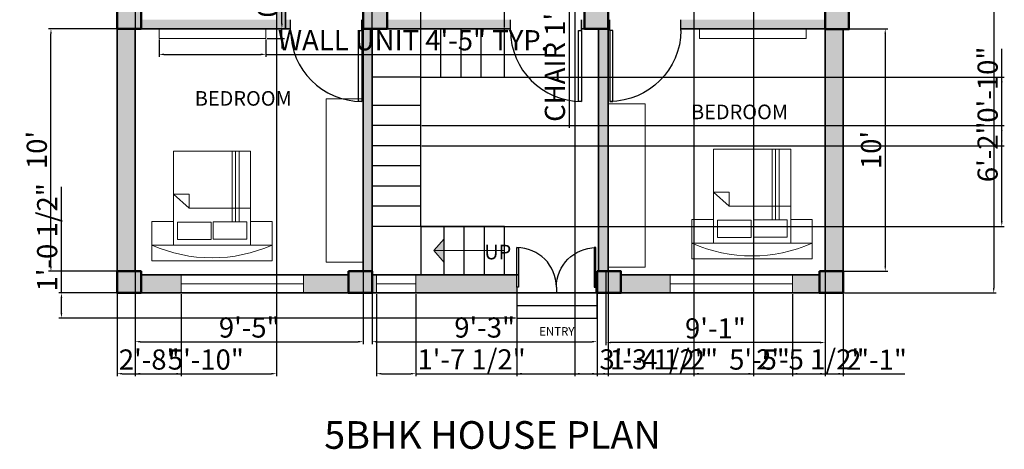
# Model space of a CAD drawing. Units: inches. Extents: x 2312 to 2808, y 1290 to 1909.
# Tile 1 of 5: x 2312 to 2800, y 1290 to 1503. Entities that reach past the tile are written whole.
import ezdxf

# ---------------------------------------------------------------- set-up
doc = ezdxf.new("R2010")
doc.units = ezdxf.units.IN
for name, color, linetype, lineweight in [('A-ANNO-DIMS', 2, 'Continuous', 18), ('A-ANNO-SYMB', 181, 'Continuous', 18), ('A-ANNO-TEXT', 7, 'Continuous', 25), ('A-AREA-IDEN', 7, 'Continuous', 25), ('A-COLS-PATT', 1, 'Continuous', 13), ('A-FLOR-CASE', 181, 'Continuous', 20), ('A-FLOR-STRS', 181, 'Continuous', 25), ('A-WALL-PATT', 150, 'Continuous', 13), ('COLUMN', 1, 'Continuous', 50), ('DOOR', 50, 'Continuous', 25), ('FUR', 130, 'Continuous', 18), ('WALL', 7, 'Continuous', 35), ('WINDOW', 70, 'Continuous', 18)]:
    doc.layers.add(name, color=color, linetype=linetype, lineweight=lineweight)
doc.styles.get("Standard").update_dxf_attribs({"font": 'arial.ttf'})
doc.dimstyles.new('ISO-25', dxfattribs={"dimtxt": 10, "dimasz": 2.5, "dimexe": 1.25, "dimexo": 0.625, "dimtad": 1, "dimdec": 0, "dimlunit": 4, "dimtxsty": 'Standard', "dimcen": 2.5, "dimadec": 0, "dimazin": 0, "dimtfac": 1, "dimtdec": 0, "dimtmove": 0, "dimatfit": 3, "dimfxl": 1, "dimarcsym": 0})

# ---------------------------------------------------------------- blocks, each defined once
blk = doc.blocks.new('*U2')
for p, q in [((0, 0), (0, -6)), ((40, 0), (40, -6))]:
    blk.add_line(p, q)
blk.add_lwpolyline([(0, 0), (0, 40), (1.75, 40), (1.75, 0)], close=True)
blk.add_arc((0, 0), 40, 0, 90)
blk = doc.blocks.new('*D6')
at = {"layer": 'A-ANNO-DIMS', "color": 0, "lineweight": -2, "transparency": 16777216}
for p, q in [((2721.06, 1775.72), (2796.28, 1775.72)), ((2795.03, 1773.22), (2795.03, 1370.22)), ((2721.06, 1367.72), (2796.28, 1367.72))]:
    blk.add_line(p, q, dxfattribs=at)
at = {"layer": 'A-ANNO-DIMS', "color": 0, "transparency": 16777216}
for points in [[(2794.62, 1773.22), (2795.45, 1773.22), (2795.03, 1775.72)], [(2794.62, 1370.22), (2795.45, 1370.22), (2795.03, 1367.72)]]:
    blk.add_solid(points, dxfattribs=at)
at = {"layer": 'Defpoints', "color": 0, "transparency": 16777216}
for p in [(2720.43, 1775.72), (2720.43, 1367.72), (2795.03, 1367.72)]:
    blk.add_point(p, dxfattribs=at)
at = {"layer": 'A-ANNO-DIMS', "color": 0, "transparency": 16777216, "insert": (2789.3, 1571.72), "char_height": 10, "attachment_point": 5, "rotation": 90}
blk.add_mtext("34'", dxfattribs=at)
blk = doc.blocks.new('*D15')
at = {"layer": 'A-ANNO-DIMS', "color": 0, "lineweight": -2, "transparency": 16777216}
for p, q in [((2712.06, 1498.72), (2742.51, 1498.72)), ((2741.26, 1496.22), (2741.26, 1380.99)), ((2712.06, 1378.49), (2742.51, 1378.49))]:
    blk.add_line(p, q, dxfattribs=at)
at = {"layer": 'A-ANNO-DIMS', "color": 0, "transparency": 16777216}
for points in [[(2740.85, 1496.22), (2741.68, 1496.22), (2741.26, 1498.72)], [(2740.85, 1380.99), (2741.68, 1380.99), (2741.26, 1378.49)]]:
    blk.add_solid(points, dxfattribs=at)
at = {"layer": 'Defpoints', "color": 0, "transparency": 16777216}
for p in [(2711.43, 1498.72), (2711.43, 1378.49), (2741.26, 1378.49)]:
    blk.add_point(p, dxfattribs=at)
at = {"layer": 'A-ANNO-DIMS', "color": 0, "transparency": 16777216, "insert": (2735.53, 1438.61), "char_height": 10, "attachment_point": 5, "rotation": 90}
blk.add_mtext("10'", dxfattribs=at)
blk = doc.blocks.new('*D16')
at = {"layer": 'A-ANNO-DIMS', "color": 0, "lineweight": -2, "transparency": 16777216}
for p, q in [((2602.69, 1377.87), (2602.69, 1341.91)), ((2711.43, 1377.87), (2711.43, 1341.91)), ((2708.93, 1343.16), (2605.19, 1343.16))]:
    blk.add_line(p, q, dxfattribs=at)
at = {"layer": 'A-ANNO-DIMS', "color": 0, "transparency": 16777216}
for points in [[(2605.19, 1343.58), (2605.19, 1342.74), (2602.69, 1343.16)], [(2708.93, 1343.58), (2708.93, 1342.74), (2711.43, 1343.16)]]:
    blk.add_solid(points, dxfattribs=at)
at = {"layer": 'Defpoints', "color": 0, "transparency": 16777216}
for p in [(2602.69, 1378.49), (2711.43, 1378.49), (2602.69, 1343.16)]:
    blk.add_point(p, dxfattribs=at)
at = {"layer": 'A-ANNO-DIMS', "color": 0, "transparency": 16777216, "insert": (2657.06, 1348.89), "char_height": 10, "attachment_point": 5}
blk.add_mtext('9\'-1"', dxfattribs=at)
blk = doc.blocks.new('*D17')
at = {"layer": 'A-ANNO-DIMS', "color": 0, "lineweight": -2, "transparency": 16777216}
for p, q in [((2486.93, 1377.87), (2486.93, 1342.33)), ((2598.36, 1376.09), (2598.36, 1342.33)), ((2489.43, 1343.58), (2595.86, 1343.58))]:
    blk.add_line(p, q, dxfattribs=at)
at = {"layer": 'A-ANNO-DIMS', "color": 0, "transparency": 16777216}
for points in [[(2489.43, 1343.99), (2489.43, 1343.16), (2486.93, 1343.58)], [(2595.86, 1343.99), (2595.86, 1343.16), (2598.36, 1343.58)]]:
    blk.add_solid(points, dxfattribs=at)
at = {"layer": 'Defpoints', "color": 0, "transparency": 16777216}
for p in [(2486.93, 1378.49), (2598.36, 1376.72), (2598.36, 1343.58)]:
    blk.add_point(p, dxfattribs=at)
at = {"layer": 'A-ANNO-DIMS', "color": 0, "transparency": 16777216, "insert": (2542.65, 1349.31), "char_height": 10, "attachment_point": 5}
blk.add_mtext('9\'-3"', dxfattribs=at)
blk = doc.blocks.new('*D18')
at = {"layer": 'A-ANNO-DIMS', "color": 0, "lineweight": -2, "transparency": 16777216}
for p, q in [((2369.43, 1377.87), (2369.43, 1342.33)), ((2482.43, 1377.87), (2482.43, 1342.33)), ((2371.93, 1343.58), (2479.93, 1343.58))]:
    blk.add_line(p, q, dxfattribs=at)
at = {"layer": 'A-ANNO-DIMS', "color": 0, "transparency": 16777216}
for points in [[(2371.93, 1343.99), (2371.93, 1343.16), (2369.43, 1343.58)], [(2479.93, 1343.99), (2479.93, 1343.16), (2482.43, 1343.58)]]:
    blk.add_solid(points, dxfattribs=at)
at = {"layer": 'Defpoints', "color": 0, "transparency": 16777216}
for p in [(2369.43, 1378.49), (2482.43, 1378.49), (2482.43, 1343.58)]:
    blk.add_point(p, dxfattribs=at)
at = {"layer": 'A-ANNO-DIMS', "color": 0, "transparency": 16777216, "insert": (2425.93, 1349.31), "char_height": 10, "attachment_point": 5}
blk.add_mtext('9\'-5"', dxfattribs=at)
blk = doc.blocks.new('*D19')
at = {"layer": 'A-ANNO-DIMS', "color": 0, "lineweight": -2, "transparency": 16777216}
for p, q in [((2368.81, 1498.72), (2326.38, 1498.72)), ((2327.63, 1380.99), (2327.63, 1496.22)), ((2368.81, 1378.49), (2326.38, 1378.49))]:
    blk.add_line(p, q, dxfattribs=at)
at = {"layer": 'A-ANNO-DIMS', "color": 0, "transparency": 16777216}
for points in [[(2327.21, 1496.22), (2328.05, 1496.22), (2327.63, 1498.72)], [(2327.21, 1380.99), (2328.05, 1380.99), (2327.63, 1378.49)]]:
    blk.add_solid(points, dxfattribs=at)
at = {"layer": 'Defpoints', "color": 0, "transparency": 16777216}
for p in [(2327.63, 1498.72), (2369.43, 1498.72), (2369.43, 1378.49)]:
    blk.add_point(p, dxfattribs=at)
at = {"layer": 'A-ANNO-DIMS', "color": 0, "transparency": 16777216, "insert": (2321.9, 1438.61), "char_height": 10, "attachment_point": 5, "rotation": 90}
blk.add_mtext("10'", dxfattribs=at)
blk = doc.blocks.new('BED-DOUBLE')
for p, q in [((0, 46.6), (0, 54.42)), ((0, 54.42), (59.67, 54.42)), ((59.67, 54.42), (59.67, 46.6)), ((16.43, 35.15), (16.43, 0)), ((18.15, 35.15), (18.15, 0)), ((19.9, 35.15), (19.9, 0)), ((10.68, 28.37), (10.68, 28.37)), ((10.68, 28.37), (41.23, 28.37)), ((41.23, 28.37), (41.23, 21.43)), ((48.99, 21.43), (41.23, 28.37)), ((41.23, 21.43), (48.99, 21.43))]:
    blk.add_line(p, q)
for points in [[(10.68, 46.6), (0, 46.6), (0, 34.89), (10.68, 34.89)], [(10.68, 46.6), (48.99, 46.6), (48.99, 0), (10.68, 0)], [(59.67, 46.6), (48.99, 46.6), (48.99, 34.89), (59.67, 34.89)], [(12.51, 43.74), (29.18, 43.74), (29.18, 35.15), (12.51, 35.15)], [(30.28, 43.78), (46.95, 43.78), (46.95, 35.19), (30.28, 35.19)]]:
    blk.add_lwpolyline(points, close=True)
blk.add_arc((29.84, -20.26), 73.22, 65.9516, 114.0484)
blk = doc.blocks.new('BEDROOM-STORAGE')
blk.add_lwpolyline([(18.34, 80.97), (0, 80.97), (0, 0), (18.34, 0)], close=True)
blk = doc.blocks.new('BEDROOM-WALL-UNIT')
blk.add_lwpolyline([(0, 0), (52.94, 0), (52.94, 4.76), (0, 4.76)], close=True)
blk = doc.blocks.new('*D33')
at = {"layer": 'A-ANNO-DIMS', "color": 0, "lineweight": -2, "transparency": 16777216}
for p, q in [((2381.24, 1493.33), (2381.24, 1484.77)), ((2434.18, 1493.33), (2434.18, 1484.77)), ((2383.74, 1486.02), (2431.68, 1486.02)), ((2434.18, 1486.02), (2577.69, 1486.02))]:
    blk.add_line(p, q, dxfattribs=at)
at = {"layer": 'A-ANNO-DIMS', "color": 0, "transparency": 16777216}
for points in [[(2383.74, 1486.43), (2383.74, 1485.6), (2381.24, 1486.02)], [(2431.68, 1486.43), (2431.68, 1485.6), (2434.18, 1486.02)]]:
    blk.add_solid(points, dxfattribs=at)
at = {"layer": 'Defpoints', "color": 0, "transparency": 16777216}
for p in [(2381.24, 1493.96), (2434.18, 1493.96), (2434.18, 1486.02)]:
    blk.add_point(p, dxfattribs=at)
at = {"layer": 'A-ANNO-DIMS', "color": 0, "transparency": 16777216, "insert": (2507.19, 1491.73), "char_height": 10, "attachment_point": 5}
blk.add_mtext('WALL UNIT 4\'-5" TYP.', dxfattribs=at)
blk = doc.blocks.new('*D34')
at = {"layer": 'A-ANNO-DIMS', "color": 0, "lineweight": -2, "transparency": 16777216}
for p, q in [((2442.12, 1501.22), (2442.12, 1565.92)), ((2434.81, 1498.72), (2443.37, 1498.72)), ((2442.12, 1493.96), (2442.12, 1498.72)), ((2434.81, 1493.96), (2443.37, 1493.96)), ((2442.12, 1491.46), (2442.12, 1488.96))]:
    blk.add_line(p, q, dxfattribs=at)
at = {"layer": 'A-ANNO-DIMS', "color": 0, "transparency": 16777216}
for points in [[(2441.7, 1501.22), (2442.54, 1501.22), (2442.12, 1498.72)], [(2441.7, 1491.46), (2442.54, 1491.46), (2442.12, 1493.96)]]:
    blk.add_solid(points, dxfattribs=at)
at = {"layer": 'Defpoints', "color": 0, "transparency": 16777216}
for p in [(2434.18, 1498.72), (2442.12, 1498.72), (2434.18, 1493.96)]:
    blk.add_point(p, dxfattribs=at)
at = {"layer": 'A-ANNO-DIMS', "color": 0, "transparency": 16777216, "insert": (2436.39, 1534.82), "char_height": 10, "attachment_point": 5, "rotation": 90}
blk.add_mtext('0\'-5" TYP.', dxfattribs=at)
blk = doc.blocks.new('*D35')
at = {"layer": 'A-ANNO-DIMS', "color": 0, "lineweight": -2, "transparency": 16777216}
for p, q in [((2585.87, 1574.5), (2583.31, 1574.5)), ((2584.56, 1572), (2584.56, 1564.12)), ((2585.87, 1561.62), (2583.31, 1561.62)), ((2584.56, 1561.62), (2584.56, 1449.68))]:
    blk.add_line(p, q, dxfattribs=at)
at = {"layer": 'A-ANNO-DIMS', "color": 0, "transparency": 16777216}
for points in [[(2584.15, 1572), (2584.98, 1572), (2584.56, 1574.5)], [(2584.15, 1564.12), (2584.98, 1564.12), (2584.56, 1561.62)]]:
    blk.add_solid(points, dxfattribs=at)
at = {"layer": 'Defpoints', "color": 0, "transparency": 16777216}
for p in [(2586.49, 1574.5), (2584.56, 1561.62), (2586.49, 1561.62)]:
    blk.add_point(p, dxfattribs=at)
at = {"layer": 'A-ANNO-DIMS', "color": 0, "transparency": 16777216, "insert": (2578.77, 1504.4), "char_height": 10, "attachment_point": 5, "rotation": 90}
blk.add_mtext('CHAIR 1\'-1" TYP.', dxfattribs=at)
blk = doc.blocks.new('*D39')
at = {"layer": 'A-ANNO-DIMS', "color": 0, "lineweight": -2, "transparency": 16777216}
for p, q in [((2646.41, 1564.09), (2646.41, 1326.46)), ((2711.43, 1564.09), (2711.43, 1326.46)), ((2648.91, 1327.71), (2708.93, 1327.71))]:
    blk.add_line(p, q, dxfattribs=at)
at = {"layer": 'A-ANNO-DIMS', "color": 0, "transparency": 16777216}
for points in [[(2648.91, 1328.13), (2648.91, 1327.3), (2646.41, 1327.71)], [(2708.93, 1328.13), (2708.93, 1327.3), (2711.43, 1327.71)]]:
    blk.add_solid(points, dxfattribs=at)
at = {"layer": 'Defpoints', "color": 0, "transparency": 16777216}
for p in [(2646.41, 1564.72), (2711.43, 1564.72), (2711.43, 1327.71)]:
    blk.add_point(p, dxfattribs=at)
at = {"layer": 'A-ANNO-DIMS', "color": 0, "transparency": 16777216, "insert": (2678.92, 1333.42), "char_height": 10, "attachment_point": 5}
blk.add_mtext('5\'-5"', dxfattribs=at)
blk = doc.blocks.new('*D40')
at = {"layer": 'A-ANNO-DIMS', "color": 0, "lineweight": -2, "transparency": 16777216}
for p, q in [((2439.43, 1545.58), (2439.43, 1326.46)), ((2369.43, 1542.44), (2369.43, 1326.46)), ((2371.93, 1327.71), (2436.93, 1327.71))]:
    blk.add_line(p, q, dxfattribs=at)
at = {"layer": 'A-ANNO-DIMS', "color": 0, "transparency": 16777216}
for points in [[(2371.93, 1328.13), (2371.93, 1327.3), (2369.43, 1327.71)], [(2436.93, 1328.13), (2436.93, 1327.3), (2439.43, 1327.71)]]:
    blk.add_solid(points, dxfattribs=at)
at = {"layer": 'Defpoints', "color": 0, "transparency": 16777216}
for p in [(2369.43, 1543.07), (2439.43, 1546.2), (2439.43, 1327.71)]:
    blk.add_point(p, dxfattribs=at)
at = {"layer": 'A-ANNO-DIMS', "color": 0, "transparency": 16777216, "insert": (2404.43, 1333.44), "char_height": 10, "attachment_point": 5}
blk.add_mtext('5\'-10"', dxfattribs=at)
blk = doc.blocks.new('*D42')
at = {"layer": 'A-ANNO-DIMS', "color": 0, "lineweight": -2, "transparency": 16777216}
for p, q in [((2558.63, 1367.09), (2558.63, 1326.46)), ((2598.36, 1367.09), (2598.36, 1326.46)), ((2561.13, 1327.71), (2595.86, 1327.71)), ((2598.36, 1327.71), (2651.99, 1327.71))]:
    blk.add_line(p, q, dxfattribs=at)
at = {"layer": 'A-ANNO-DIMS', "color": 0, "transparency": 16777216}
for points in [[(2561.13, 1328.13), (2561.13, 1327.3), (2558.63, 1327.71)], [(2595.86, 1328.13), (2595.86, 1327.3), (2598.36, 1327.71)]]:
    blk.add_solid(points, dxfattribs=at)
at = {"layer": 'Defpoints', "color": 0, "transparency": 16777216}
for p in [(2558.63, 1367.72), (2598.36, 1367.72), (2598.36, 1327.71)]:
    blk.add_point(p, dxfattribs=at)
at = {"layer": 'A-ANNO-DIMS', "color": 0, "transparency": 16777216, "insert": (2626.42, 1333.51), "char_height": 10, "attachment_point": 5}
blk.add_mtext('3\'-3 1/2"', dxfattribs=at)
blk = doc.blocks.new('*D43')
at = {"layer": 'A-ANNO-DIMS', "color": 0, "lineweight": -2, "transparency": 16777216}
for p, q in [((2486.93, 1401.34), (2486.93, 1804.57)), ((2489.43, 1803.32), (2508.43, 1803.32)), ((2510.93, 1401.34), (2510.93, 1804.57)), ((2510.93, 1803.32), (2541.44, 1803.32))]:
    blk.add_line(p, q, dxfattribs=at)
at = {"layer": 'A-ANNO-DIMS', "color": 0, "transparency": 16777216}
for points in [[(2489.43, 1803.73), (2489.43, 1802.9), (2486.93, 1803.32)], [(2508.43, 1803.73), (2508.43, 1802.9), (2510.93, 1803.32)]]:
    blk.add_solid(points, dxfattribs=at)
at = {"layer": 'Defpoints', "color": 0, "transparency": 16777216}
for p in [(2510.93, 1803.32), (2486.93, 1400.72), (2510.93, 1400.72)]:
    blk.add_point(p, dxfattribs=at)
at = {"layer": 'A-ANNO-DIMS', "color": 0, "transparency": 16777216, "insert": (2527.44, 1809.05), "char_height": 10, "attachment_point": 5}
blk.add_mtext('2\'-0"', dxfattribs=at)
blk = doc.blocks.new('*D51')
at = {"layer": 'A-ANNO-DIMS', "color": 0, "lineweight": -2, "transparency": 16777216}
for p, q in [((2646.41, 1624.89), (2646.41, 1326.46)), ((2675.95, 1624.89), (2675.95, 1326.46)), ((2648.91, 1327.71), (2673.45, 1327.71)), ((2675.95, 1327.71), (2729.75, 1327.71))]:
    blk.add_line(p, q, dxfattribs=at)
at = {"layer": 'A-ANNO-DIMS', "color": 0, "transparency": 16777216}
for points in [[(2648.91, 1328.13), (2648.91, 1327.3), (2646.41, 1327.71)], [(2673.45, 1328.13), (2673.45, 1327.3), (2675.95, 1327.71)]]:
    blk.add_solid(points, dxfattribs=at)
at = {"layer": 'Defpoints', "color": 0, "transparency": 16777216}
for p in [(2646.41, 1625.52), (2675.95, 1625.52), (2675.95, 1327.71)]:
    blk.add_point(p, dxfattribs=at)
at = {"layer": 'A-ANNO-DIMS', "color": 0, "transparency": 16777216, "insert": (2704.1, 1333.51), "char_height": 10, "attachment_point": 5}
blk.add_mtext('2\'-5 1/2"', dxfattribs=at)
blk = doc.blocks.new('*D60')
at = {"layer": 'A-ANNO-DIMS', "color": 0, "lineweight": -2, "transparency": 16777216}
for p, q in [((2488.96, 1367.09), (2488.96, 1326.46)), ((2508.56, 1367.09), (2508.56, 1326.46)), ((2491.46, 1327.71), (2506.06, 1327.71)), ((2508.56, 1327.71), (2561.25, 1327.71))]:
    blk.add_line(p, q, dxfattribs=at)
at = {"layer": 'A-ANNO-DIMS', "color": 0, "transparency": 16777216}
for points in [[(2491.46, 1328.13), (2491.46, 1327.3), (2488.96, 1327.71)], [(2506.06, 1328.13), (2506.06, 1327.3), (2508.56, 1327.71)]]:
    blk.add_solid(points, dxfattribs=at)
at = {"layer": 'Defpoints', "color": 0, "transparency": 16777216}
for p in [(2488.96, 1367.72), (2508.56, 1367.72), (2508.56, 1327.71)]:
    blk.add_point(p, dxfattribs=at)
at = {"layer": 'A-ANNO-DIMS', "color": 0, "transparency": 16777216, "insert": (2536.16, 1333.51), "char_height": 10, "attachment_point": 5}
blk.add_mtext('1\'-7 1/2"', dxfattribs=at)
blk = doc.blocks.new('*D61')
at = {"layer": 'A-ANNO-DIMS', "color": 0, "lineweight": -2, "transparency": 16777216}
for p, q in [((2799.03, 1450.72), (2799.03, 1488.82)), ((2511.56, 1450.72), (2800.28, 1450.72)), ((2799.03, 1443.22), (2799.03, 1448.22)), ((2511.56, 1440.72), (2800.28, 1440.72))]:
    blk.add_line(p, q, dxfattribs=at)
at = {"layer": 'A-ANNO-DIMS', "color": 0, "transparency": 16777216}
for points in [[(2798.62, 1448.22), (2799.45, 1448.22), (2799.03, 1450.72)], [(2798.62, 1443.22), (2799.45, 1443.22), (2799.03, 1440.72)]]:
    blk.add_solid(points, dxfattribs=at)
at = {"layer": 'Defpoints', "color": 0, "transparency": 16777216}
for p in [(2510.93, 1450.72), (2799.03, 1450.72), (2510.93, 1440.72)]:
    blk.add_point(p, dxfattribs=at)
at = {"layer": 'A-ANNO-DIMS', "color": 0, "transparency": 16777216, "insert": (2793.3, 1471.02), "char_height": 10, "attachment_point": 5, "rotation": 90}
blk.add_mtext('0\'-10"', dxfattribs=at)
blk = doc.blocks.new('*D66')
at = {"layer": 'A-ANNO-DIMS', "color": 0, "lineweight": -2, "transparency": 16777216}
for p, q in [((2332.83, 1367.72), (2332.83, 1420.41)), ((2558, 1367.72), (2331.58, 1367.72)), ((2332.83, 1357.81), (2332.83, 1365.22)), ((2558, 1355.31), (2331.58, 1355.31))]:
    blk.add_line(p, q, dxfattribs=at)
at = {"layer": 'A-ANNO-DIMS', "color": 0, "transparency": 16777216}
for points in [[(2332.42, 1365.22), (2333.25, 1365.22), (2332.83, 1367.72)], [(2332.42, 1357.81), (2333.25, 1357.81), (2332.83, 1355.31)]]:
    blk.add_solid(points, dxfattribs=at)
at = {"layer": 'Defpoints', "color": 0, "transparency": 16777216}
for p in [(2332.83, 1367.72), (2558.63, 1367.72), (2558.63, 1355.31)]:
    blk.add_point(p, dxfattribs=at)
at = {"layer": 'A-ANNO-DIMS', "color": 0, "transparency": 16777216, "insert": (2327.04, 1395.31), "char_height": 10, "attachment_point": 5, "rotation": 90}
blk.add_mtext('1\'-0 1/2"', dxfattribs=at)
blk = doc.blocks.new('*D67')
at = {"layer": 'A-ANNO-DIMS', "color": 0, "lineweight": -2, "transparency": 16777216}
for p, q in [((2486.93, 1499.34), (2486.93, 1804.57)), ((2489.43, 1803.32), (2550.01, 1803.32)), ((2552.51, 1499.34), (2552.51, 1804.57))]:
    blk.add_line(p, q, dxfattribs=at)
at = {"layer": 'A-ANNO-DIMS', "color": 0, "transparency": 16777216}
for points in [[(2489.43, 1803.73), (2489.43, 1802.9), (2486.93, 1803.32)], [(2550.01, 1803.73), (2550.01, 1802.9), (2552.51, 1803.32)]]:
    blk.add_solid(points, dxfattribs=at)
at = {"layer": 'Defpoints', "color": 0, "transparency": 16777216}
for p in [(2552.51, 1803.32), (2486.93, 1498.72), (2552.51, 1498.72)]:
    blk.add_point(p, dxfattribs=at)
at = {"layer": 'A-ANNO-DIMS', "color": 0, "transparency": 16777216, "insert": (2519.72, 1809.11), "char_height": 10, "attachment_point": 5}
blk.add_mtext('5\'-5 1/2"', dxfattribs=at)
blk = doc.blocks.new('*D68')
at = {"layer": 'A-ANNO-DIMS', "color": 0, "lineweight": -2, "transparency": 16777216}
for p, q in [((2511.56, 1474.72), (2800.28, 1474.72)), ((2799.03, 1403.22), (2799.03, 1472.22)), ((2511.56, 1400.72), (2800.28, 1400.72))]:
    blk.add_line(p, q, dxfattribs=at)
at = {"layer": 'A-ANNO-DIMS', "color": 0, "transparency": 16777216}
for points in [[(2798.62, 1472.22), (2799.45, 1472.22), (2799.03, 1474.72)], [(2798.62, 1403.22), (2799.45, 1403.22), (2799.03, 1400.72)]]:
    blk.add_solid(points, dxfattribs=at)
at = {"layer": 'Defpoints', "color": 0, "transparency": 16777216}
for p in [(2510.93, 1474.72), (2799.03, 1474.72), (2510.93, 1400.72)]:
    blk.add_point(p, dxfattribs=at)
at = {"layer": 'A-ANNO-DIMS', "color": 0, "transparency": 16777216, "insert": (2793.3, 1437.72), "char_height": 10, "attachment_point": 5, "rotation": 90}
blk.add_mtext('6\'-2"', dxfattribs=at)
blk = doc.blocks.new('*D69')
at = {"layer": 'A-ANNO-DIMS', "color": 0, "lineweight": -2, "transparency": 16777216}
for p, q in [((2360.43, 1367.09), (2360.43, 1326.46)), ((2392.25, 1367.09), (2392.25, 1326.46)), ((2362.93, 1327.71), (2389.75, 1327.71))]:
    blk.add_line(p, q, dxfattribs=at)
at = {"layer": 'A-ANNO-DIMS', "color": 0, "transparency": 16777216}
for points in [[(2362.93, 1328.13), (2362.93, 1327.3), (2360.43, 1327.71)], [(2389.75, 1328.13), (2389.75, 1327.3), (2392.25, 1327.71)]]:
    blk.add_solid(points, dxfattribs=at)
at = {"layer": 'Defpoints', "color": 0, "transparency": 16777216}
for p in [(2360.43, 1367.72), (2392.25, 1367.72), (2392.25, 1327.71)]:
    blk.add_point(p, dxfattribs=at)
at = {"layer": 'A-ANNO-DIMS', "color": 0, "transparency": 16777216, "insert": (2376.34, 1333.44), "char_height": 10, "attachment_point": 5}
blk.add_mtext('2\'-8"', dxfattribs=at)
blk = doc.blocks.new('*D70')
at = {"layer": 'A-ANNO-DIMS', "color": 0, "lineweight": -2, "transparency": 16777216}
for p, q in [((2695.25, 1367.09), (2695.25, 1326.46)), ((2720.43, 1367.09), (2720.43, 1326.46)), ((2697.75, 1327.71), (2717.93, 1327.71)), ((2720.43, 1327.71), (2750.94, 1327.71))]:
    blk.add_line(p, q, dxfattribs=at)
at = {"layer": 'A-ANNO-DIMS', "color": 0, "transparency": 16777216}
for points in [[(2697.75, 1328.13), (2697.75, 1327.3), (2695.25, 1327.71)], [(2717.93, 1328.13), (2717.93, 1327.3), (2720.43, 1327.71)]]:
    blk.add_solid(points, dxfattribs=at)
at = {"layer": 'Defpoints', "color": 0, "transparency": 16777216}
for p in [(2695.25, 1367.72), (2720.43, 1367.72), (2720.43, 1327.71)]:
    blk.add_point(p, dxfattribs=at)
at = {"layer": 'A-ANNO-DIMS', "color": 0, "transparency": 16777216, "insert": (2736.94, 1333.36), "char_height": 10, "attachment_point": 5}
blk.add_mtext('2\'-1"', dxfattribs=at)
blk = doc.blocks.new('*D71')
at = {"layer": 'A-ANNO-DIMS', "color": 0, "lineweight": -2, "transparency": 16777216}
for p, q in [((2587.32, 1629.59), (2587.32, 1326.46)), ((2603.93, 1629.59), (2603.93, 1326.46)), ((2589.82, 1327.71), (2601.43, 1327.71)), ((2603.93, 1327.71), (2656.63, 1327.71))]:
    blk.add_line(p, q, dxfattribs=at)
at = {"layer": 'A-ANNO-DIMS', "color": 0, "transparency": 16777216}
for points in [[(2589.82, 1328.13), (2589.82, 1327.3), (2587.32, 1327.71)], [(2601.43, 1328.13), (2601.43, 1327.3), (2603.93, 1327.71)]]:
    blk.add_solid(points, dxfattribs=at)
at = {"layer": 'Defpoints', "color": 0, "transparency": 16777216}
for p in [(2587.32, 1630.22), (2603.93, 1630.22), (2603.93, 1327.71)]:
    blk.add_point(p, dxfattribs=at)
at = {"layer": 'A-ANNO-DIMS', "color": 0, "transparency": 16777216, "insert": (2631.53, 1333.51), "char_height": 10, "attachment_point": 5}
blk.add_mtext('1\'-4 1/2"', dxfattribs=at)

msp = doc.modelspace()

# ---------------------------------------------------------------- hatches: boundary and pattern name
at = {"layer": 'A-ANNO-SYMB'}
h = msp.add_hatch(color=256, dxfattribs=at)
h.dxf.hatch_style = 1
h.paths.add_polyline_path([(2522.51, 1388.72), (2517.41, 1388.72), (2522.51, 1382.91)])
h.paths.add_polyline_path([(2522.51, 1394.52), (2517.41, 1388.72), (2522.51, 1388.72)])
at = {"layer": 'A-COLS-PATT'}
h = msp.add_hatch(color=256, dxfattribs=at)
h.dxf.hatch_style = 1
h.paths.add_polyline_path([(2372.28, 1775.72), (2360.43, 1775.72), (2360.43, 1764.94), (2372.28, 1764.94)])
h.paths.add_polyline_path([(2486.97, 1775.72), (2475.12, 1775.72), (2475.12, 1764.94), (2486.93, 1764.94), (2486.93, 1766.72)])
h.paths.add_polyline_path([(2610.92, 1775.72), (2599.07, 1775.72), (2599.07, 1766.72), (2599.11, 1766.72), (2599.11, 1764.94), (2610.92, 1764.94)])
h.paths.add_polyline_path([(2720.43, 1775.72), (2708.59, 1775.72), (2708.59, 1764.94), (2720.43, 1764.94)])
h.paths.add_polyline_path([(2723.28, 1640.11), (2711.43, 1640.11), (2711.43, 1629.34), (2723.28, 1629.34)])
h.paths.add_polyline_path([(2603.61, 1640.99), (2592.09, 1640.99), (2592.09, 1630.22), (2603.93, 1630.22), (2603.93, 1634.72), (2603.61, 1634.72)])
h.paths.add_polyline_path([(2494.28, 1640.99), (2482.43, 1640.99), (2482.43, 1630.22), (2494.28, 1630.22)])
h.paths.add_polyline_path([(2372.28, 1640.99), (2360.43, 1640.99), (2360.43, 1630.22), (2372.28, 1630.22)])
h.paths.add_polyline_path([(2372.28, 1509.49), (2360.43, 1509.49), (2360.43, 1498.72), (2372.28, 1498.72)])
h.paths.add_polyline_path([(2494.28, 1509.49), (2482.43, 1509.49), (2482.43, 1498.72), (2494.28, 1498.72)])
h.paths.add_polyline_path([(2603.93, 1509.49), (2592.09, 1509.49), (2592.09, 1498.72), (2603.93, 1498.72)])
h.paths.add_polyline_path([(2723.28, 1509.26), (2711.43, 1509.26), (2711.43, 1498.48), (2723.28, 1498.48)])
h.paths.add_polyline_path([(2720.43, 1378.49), (2708.59, 1378.49), (2708.59, 1367.72), (2720.43, 1367.72)])
h.paths.add_polyline_path([(2610.2, 1378.49), (2598.36, 1378.49), (2598.36, 1367.72), (2610.2, 1367.72)])
h.paths.add_polyline_path([(2486.94, 1376.72), (2486.93, 1376.72), (2486.93, 1378.49), (2475.1, 1378.49), (2475.1, 1367.72), (2486.94, 1367.72)])
h.paths.add_polyline_path([(2372.28, 1378.49), (2360.43, 1378.49), (2360.43, 1367.72), (2372.28, 1367.72)])
at = {"layer": 'A-WALL-PATT'}
h = msp.add_hatch(color=256, dxfattribs=at)
h.dxf.hatch_style = 1
h.paths.add_polyline_path([(2369.43, 1764.94), (2360.43, 1764.94), (2360.43, 1640.99), (2369.43, 1640.99)])
h.paths.add_polyline_path([(2720.43, 1764.94), (2711.43, 1764.94), (2711.43, 1640.11), (2720.43, 1640.11)])
h.paths.add_polyline_path([(2552.09, 1634.72), (2494.28, 1634.72), (2494.28, 1630.22), (2552.09, 1630.22)])
h.paths.add_polyline_path([(2446.36, 1634.72), (2372.28, 1634.72), (2372.28, 1630.22), (2405.43, 1630.22), (2439.43, 1630.22), (2446.36, 1630.22)])
h.paths.add_polyline_path([(2443.93, 1630.22), (2439.43, 1630.22), (2439.43, 1596.05), (2443.93, 1596.05)])
h.paths.add_polyline_path([(2486.93, 1630.22), (2482.43, 1630.22), (2482.43, 1509.49), (2486.93, 1509.49)])
h.paths.add_polyline_path([(2443.93, 1546.2), (2439.43, 1546.2), (2439.43, 1503.22), (2372.28, 1503.22), (2372.28, 1498.72), (2443.93, 1498.72)])
h.paths.add_polyline_path([(2555.45, 1503.22), (2494.28, 1503.22), (2494.28, 1498.72), (2555.45, 1498.72)])
h.paths.add_polyline_path([(2711.43, 1503.22), (2639.88, 1503.22), (2639.88, 1498.72), (2711.43, 1498.72)])
h.paths.add_polyline_path([(2646.41, 1564.72), (2711.43, 1564.72), (2711.43, 1569.22), (2646.41, 1569.22), (2646.41, 1597.21), (2641.91, 1597.21), (2641.91, 1564.72), (2641.91, 1536.48), (2646.41, 1536.48)])
h.paths.add_polyline_path([(2720.43, 1498.48), (2711.43, 1498.48), (2711.43, 1378.49), (2720.43, 1378.49)])
h.paths.add_polyline_path([(2369.43, 1498.72), (2360.43, 1498.72), (2360.43, 1378.49), (2369.43, 1378.49)])
h.paths.add_polyline_path([(2486.93, 1498.72), (2482.43, 1498.72), (2482.43, 1378.49), (2486.93, 1378.49)])
h.paths.add_polyline_path([(2603.93, 1498.72), (2599.11, 1498.72), (2599.11, 1378.49), (2603.93, 1378.49)])
h.paths.add_polyline_path([(2510.36, 1766.72), (2510.36, 1775.72), (2486.97, 1775.72), (2486.97, 1766.72)])
h.paths.add_polyline_path([(2571.02, 1775.72), (2571.02, 1766.72), (2599.07, 1766.72), (2599.07, 1775.72)])
h.paths.add_polyline_path([(2393.8, 1766.72), (2393.8, 1775.72), (2372.28, 1775.72), (2372.28, 1766.72)])
h.paths.add_polyline_path([(2454.45, 1775.72), (2454.45, 1766.72), (2475.12, 1766.72), (2475.12, 1775.72)])
h.paths.add_polyline_path([(2694.96, 1775.72), (2694.96, 1766.72), (2708.59, 1766.72), (2708.59, 1775.72)])
h.paths.add_polyline_path([(2634.31, 1766.72), (2634.31, 1775.72), (2610.92, 1775.72), (2610.92, 1766.72)])
h.paths.add_polyline_path([(2392.25, 1367.72), (2392.25, 1376.72), (2372.28, 1376.72), (2372.28, 1367.72)])
h.paths.add_polyline_path([(2452.9, 1376.72), (2452.9, 1367.72), (2475.1, 1367.72), (2475.1, 1376.72)])
h.paths.add_polyline_path([(2508.56, 1376.72), (2508.56, 1367.72), (2558.63, 1367.72), (2558.63, 1370.65), (2558.63, 1376.72)])
h.paths.add_polyline_path([(2488.96, 1367.72), (2488.96, 1376.72), (2486.94, 1376.72), (2486.94, 1367.72)])
h.paths.add_polyline_path([(2634.6, 1367.72), (2634.6, 1376.72), (2610.2, 1376.72), (2610.2, 1367.72)])
h.paths.add_polyline_path([(2695.25, 1376.72), (2695.25, 1367.72), (2708.59, 1367.72), (2708.59, 1376.72)])
h.paths.add_polyline_path([(2360.43, 1590.4), (2369.43, 1590.4), (2369.43, 1630.22), (2360.43, 1630.22)])
h.paths.add_polyline_path([(2369.43, 1543.07), (2360.43, 1543.07), (2360.43, 1509.49), (2369.43, 1509.49)])
h.paths.add_polyline_path([(2720.43, 1531.67), (2711.43, 1531.67), (2711.43, 1509.26), (2720.43, 1509.26)])
h.paths.add_polyline_path([(2720.43, 1572.68), (2711.43, 1572.68), (2711.43, 1558.71), (2720.43, 1558.71)])
h.paths.add_polyline_path([(2711.43, 1599.72), (2720.43, 1599.72), (2720.43, 1629.34), (2711.43, 1629.34)])
h = msp.add_hatch(color=256, dxfattribs=at)
h.dxf.hatch_style = 1
h.paths.add_polyline_path([(2446.46, 1503.22), (2443.93, 1503.22), (2443.93, 1498.72), (2446.46, 1498.72)])
h.paths.add_polyline_path([(2482.43, 1503.22), (2481.69, 1503.22), (2481.69, 1498.72), (2482.43, 1498.72)])
h.paths.add_polyline_path([(2592.09, 1503.22), (2590.68, 1503.22), (2590.68, 1498.72), (2592.09, 1498.72)])
h.paths.add_polyline_path([(2604.66, 1503.22), (2603.93, 1503.22), (2603.93, 1498.72), (2604.66, 1498.72)])

# ---------------------------------------------------------------- linework, layer by layer
at = {"layer": 'A-ANNO-SYMB'}
for p, q in [((2517.41, 1388.72), (2522.51, 1394.52)), ((2552.51, 1388.72), (2517.41, 1388.72)), ((2517.41, 1388.72), (2522.51, 1382.91))]:
    msp.add_line(p, q, dxfattribs=at)
at = {"layer": 'A-FLOR-STRS'}
for p, q in [((2510.93, 1474.72), (2510.93, 1498.72)), ((2520.93, 1474.72), (2520.93, 1498.72)), ((2530.93, 1474.72), (2530.93, 1498.72)), ((2540.93, 1474.72), (2540.93, 1498.72)), ((2552.51, 1474.72), (2552.51, 1498.72)), ((2510.93, 1474.72), (2486.93, 1474.72)), ((2510.93, 1400.72), (2510.93, 1474.72)), ((2510.93, 1474.72), (2552.51, 1474.72)), ((2510.93, 1460.72), (2486.93, 1460.72)), ((2510.93, 1450.72), (2486.93, 1450.72)), ((2510.93, 1440.72), (2486.93, 1440.72)), ((2510.93, 1430.72), (2486.93, 1430.72)), ((2510.93, 1420.72), (2486.93, 1420.72)), ((2510.93, 1410.72), (2486.93, 1410.72)), ((2510.93, 1400.72), (2486.93, 1400.72)), ((2512.75, 1400.72), (2510.93, 1400.72)), ((2510.93, 1400.72), (2510.93, 1376.72)), ((2552.51, 1400.72), (2512.75, 1400.72)), ((2522.51, 1376.72), (2522.51, 1400.72)), ((2532.51, 1376.72), (2532.51, 1400.72)), ((2542.51, 1376.72), (2542.51, 1400.72)), ((2552.51, 1376.72), (2552.51, 1400.72)), ((2558.63, 1367.72), (2558.63, 1355.31)), ((2598.36, 1355.31), (2598.36, 1367.72)), ((2558.63, 1361.51), (2598.36, 1361.51)), ((2558.63, 1355.31), (2598.36, 1355.31))]:
    msp.add_line(p, q, dxfattribs=at)
at = {"layer": 'COLUMN'}
for points in [[(2360.43, 1509.49), (2372.28, 1509.49), (2372.28, 1498.72), (2360.43, 1498.72)], [(2482.43, 1509.49), (2494.28, 1509.49), (2494.28, 1498.72), (2482.43, 1498.72)], [(2592.09, 1509.49), (2603.93, 1509.49), (2603.93, 1498.72), (2592.09, 1498.72)], [(2711.43, 1509.26), (2723.28, 1509.26), (2723.28, 1498.48), (2711.43, 1498.48)], [(2360.43, 1378.49), (2372.28, 1378.49), (2372.28, 1367.72), (2360.43, 1367.72)], [(2475.1, 1378.49), (2486.94, 1378.49), (2486.94, 1367.72), (2475.1, 1367.72)], [(2598.36, 1378.49), (2610.2, 1378.49), (2610.2, 1367.72), (2598.36, 1367.72)], [(2708.59, 1378.49), (2720.43, 1378.49), (2720.43, 1367.72), (2708.59, 1367.72)]]:
    msp.add_lwpolyline(points, close=True, dxfattribs=at)
at = {"layer": 'WALL'}
for p, q in [((2360.43, 1367.72), (2360.43, 1775.72)), ((2482.43, 1634.72), (2482.43, 1378.49)), ((2443.93, 1546.2), (2443.93, 1498.72)), ((2443.93, 1498.72), (2369.43, 1498.72)), ((2443.93, 1498.72), (2446.46, 1498.72)), ((2481.69, 1498.72), (2555.45, 1498.72)), ((2486.93, 1498.72), (2486.93, 1376.72)), ((2590.68, 1498.72), (2604.66, 1498.72)), ((2599.11, 1498.72), (2599.11, 1378.49)), ((2603.93, 1503.22), (2603.93, 1378.49)), ((2639.88, 1498.72), (2711.43, 1498.72)), ((2720.43, 1498.48), (2720.43, 1367.72)), ((2708.59, 1376.72), (2610.2, 1376.72)), ((2720.43, 1367.72), (2360.43, 1367.72))]:
    msp.add_line(p, q, dxfattribs=at)
for points in [[(2720.43, 1498.48), (2720.43, 1367.72), (2360.43, 1367.72), (2360.43, 1775.72), (2720.43, 1775.72), (2720.43, 1640.11)], [(2711.43, 1764.94), (2711.43, 1378.49)], [(2369.43, 1378.49), (2369.43, 1498.72)], [(2475.1, 1376.72), (2372.28, 1376.72)], [(2559.48, 1376.72), (2486.93, 1376.72)], [(2598.36, 1376.72), (2596.89, 1376.72)], [(2708.59, 1376.72), (2610.2, 1376.72)]]:
    msp.add_lwpolyline(points, dxfattribs=at)
at = {"layer": 'WINDOW'}
for p, q in [((2392.25, 1372.22), (2452.9, 1372.22)), ((2488.96, 1372.22), (2508.56, 1372.22)), ((2634.6, 1372.22), (2695.25, 1372.22))]:
    msp.add_line(p, q, dxfattribs=at)
for points in [[(2392.25, 1376.72), (2452.9, 1376.72), (2452.9, 1367.72), (2392.25, 1367.72)], [(2488.96, 1376.72), (2508.56, 1376.72), (2508.56, 1367.72), (2488.96, 1367.72)], [(2634.6, 1376.72), (2695.25, 1376.72), (2695.25, 1367.72), (2634.6, 1367.72)]]:
    msp.add_lwpolyline(points, close=True, dxfattribs=at)

# ---------------------------------------------------------------- block references
at = {"layer": 'A-FLOR-CASE'}
for name, p in [('BEDROOM-WALL-UNIT', (2381.24, 1493.96)), ('BEDROOM-WALL-UNIT', (2649.12, 1493.96)), ('BEDROOM-STORAGE', (2464.09, 1383.02)), ('BEDROOM-STORAGE', (2603.93, 1380.49))]:
    msp.add_blockref(name, p, dxfattribs=at)
at = {"layer": 'DOOR', "yscale": 0.8806546932443936, "zscale": 0.8806546932443936, "rotation": 180}
for p, xscale in [((2481.69, 1497.93), 0.8806546932443936), ((2590.68, 1497.93), 0.8806546932443936), ((2604.66, 1497.93), -0.8806546932443936)]:
    msp.add_blockref('*U2', p, dxfattribs=dict(at, xscale=xscale))
at = {"layer": 'DOOR', "yscale": 0.4890082417773931, "zscale": 0.4890082417773931}
for p, xscale in [((2558.63, 1370.65), 0.4890082417773931), ((2597.75, 1370.65), -0.4890082417773931)]:
    msp.add_blockref('*U2', p, dxfattribs=dict(at, xscale=xscale))
at = {"layer": 'FUR', "rotation": 180}
for p in [(2437.31, 1438.1), (2705.06, 1439.07)]:
    msp.add_blockref('BED-DOUBLE', p, dxfattribs=at)

# ---------------------------------------------------------------- texts
at = {"layer": 'A-ANNO-TEXT', "attachment_point": 1}
for s, width, gutter_width, insert, char_height in [('UP', 196.5617, 36.22, (2542.46, 1391.64), 7.244), ('ENTRY', 112.7658, 20.78, (2569.7, 1350.79), 4.156), ('5BHK HOUSE PLAN', 2414.0778, 68.56, (2463.11, 1304.18), 13.7119)]:
    msp.add_mtext_dynamic_manual_height_columns(s, width=width, gutter_width=gutter_width, heights=[0], dxfattribs=dict(at, insert=insert, char_height=char_height))
at = {"layer": 'A-AREA-IDEN', "char_height": 7.244, "attachment_point": 1}
for insert in [(2398.94, 1467.82), (2644.98, 1461.12)]:
    msp.add_mtext_dynamic_manual_height_columns('BEDROOM', width=196.5617, gutter_width=36.22, heights=[0], dxfattribs=dict(at, insert=insert))

# ---------------------------------------------------------------- dimensions: what is measured, and where the dimension line sits
at = {"layer": 'A-ANNO-DIMS'}
for base, p1, p2, override, picture, middle in [((2552.51, 1803.32), (2486.93, 1498.72), (2552.51, 1498.72), {"dimdec": 1, "dimlfac": 1, "dimrnd": 0, "dimzin": 1, "dimdsep": 46, "dimlunit": 4, "dimfrac": 2}, '*D67', (2519.72, 1809.11)), ((2510.93, 1803.32), (2486.93, 1400.72), (2510.93, 1400.72), {"dimdec": 1, "dimlfac": 1, "dimrnd": 0, "dimzin": 1, "dimdsep": 46, "dimlunit": 4, "dimfrac": 2}, '*D43', (2527.44, 1809.05)), ((2603.93, 1327.71), (2587.32, 1630.22), (2603.93, 1630.22), {"dimdec": 1, "dimlfac": 1, "dimrnd": 0, "dimzin": 1, "dimdsep": 46, "dimlunit": 4, "dimfrac": 2}, '*D71', (2631.53, 1333.51)), ((2675.95, 1327.71), (2646.41, 1625.52), (2675.95, 1625.52), {"dimdec": 1, "dimlfac": 1, "dimrnd": 0, "dimzin": 1, "dimdsep": 46, "dimlunit": 4, "dimfrac": 2}, '*D51', (2704.1, 1333.51)), ((2711.43, 1327.71), (2646.41, 1564.72), (2711.43, 1564.72), {"dimdec": 1, "dimlfac": 1, "dimrnd": 0, "dimzin": 1, "dimdsep": 46, "dimlunit": 4, "dimfrac": 2}, '*D39', (2678.92, 1333.42)), ((2439.43, 1327.71), (2369.43, 1543.07), (2439.43, 1546.2), {"dimdec": 1, "dimlfac": 1, "dimrnd": 0, "dimzin": 1, "dimdsep": 46, "dimlunit": 4, "dimfrac": 2}, '*D40', (2404.43, 1333.44)), ((2482.43, 1343.58), (2369.43, 1378.49), (2482.43, 1378.49), {"dimclrd": 0, "dimclre": 0, "dimclrt": 0}, '*D18', (2425.93, 1349.31)), ((2598.36, 1343.58), (2486.93, 1378.49), (2598.36, 1376.72), {"dimclrd": 0, "dimclre": 0, "dimclrt": 0}, '*D17', (2542.65, 1349.31)), ((2602.69, 1343.16), (2711.43, 1378.49), (2602.69, 1378.49), {"dimclrd": 0, "dimclre": 0, "dimclrt": 0}, '*D16', (2657.06, 1348.89)), ((2392.25, 1327.71), (2360.43, 1367.72), (2392.25, 1367.72), {"dimdec": 1, "dimlfac": 1, "dimrnd": 0, "dimzin": 1, "dimdsep": 46, "dimlunit": 4, "dimfrac": 2}, '*D69', (2376.34, 1333.44)), ((2508.56, 1327.71), (2488.96, 1367.72), (2508.56, 1367.72), {"dimdec": 1, "dimlfac": 1, "dimrnd": 0, "dimzin": 1, "dimdsep": 46, "dimlunit": 4, "dimfrac": 2}, '*D60', (2536.16, 1333.51)), ((2598.36, 1327.71), (2558.63, 1367.72), (2598.36, 1367.72), {"dimdec": 1, "dimlfac": 1, "dimrnd": 0, "dimzin": 1, "dimdsep": 46, "dimlunit": 4, "dimfrac": 2}, '*D42', (2626.42, 1333.51)), ((2720.43, 1327.71), (2695.25, 1367.72), (2720.43, 1367.72), {"dimdec": 1, "dimlfac": 1, "dimrnd": 0, "dimzin": 1, "dimdsep": 46, "dimlunit": 4, "dimfrac": 2}, '*D70', (2736.94, 1333.36))]:
    dim = msp.add_linear_dim(base=base, p1=p1, p2=p2, dimstyle='ISO-25', override=override, dxfattribs=at)
    dim.commit()
    dim.dimension.update_dxf_attribs({"geometry": picture, "text_midpoint": middle})
for base, p1, p2, override, picture, middle in [((2795.03, 1367.72), (2720.43, 1775.72), (2720.43, 1367.72), {"dimclrd": 0, "dimclre": 0, "dimclrt": 0}, '*D6', (2789.3, 1571.72)), ((2327.63, 1498.72), (2369.43, 1378.49), (2369.43, 1498.72), {"dimclrd": 0, "dimclre": 0, "dimclrt": 0}, '*D19', (2321.9, 1438.61)), ((2741.26, 1378.49), (2711.43, 1498.72), (2711.43, 1378.49), {"dimclrd": 0, "dimclre": 0, "dimclrt": 0}, '*D15', (2735.53, 1438.61)), ((2799.03, 1450.72), (2510.93, 1440.72), (2510.93, 1450.72), {"dimdec": 1, "dimlfac": 1, "dimrnd": 0, "dimzin": 1, "dimdsep": 46, "dimlunit": 4, "dimfrac": 2}, '*D61', (2793.3, 1471.02)), ((2799.03, 1474.72), (2510.93, 1400.72), (2510.93, 1474.72), {"dimdec": 1, "dimlfac": 1, "dimrnd": 0, "dimzin": 1, "dimdsep": 46, "dimlunit": 4, "dimfrac": 2}, '*D68', (2793.3, 1437.72)), ((2332.83, 1367.72), (2558.63, 1355.31), (2558.63, 1367.72), {"dimdec": 1, "dimlfac": 1, "dimrnd": 0, "dimzin": 1, "dimdsep": 46, "dimlunit": 4, "dimfrac": 2}, '*D66', (2327.04, 1395.31))]:
    dim = msp.add_linear_dim(base=base, p1=p1, p2=p2, angle=90, dimstyle='ISO-25', override=override, dxfattribs=at)
    dim.commit()
    dim.dimension.update_dxf_attribs({"geometry": picture, "text_midpoint": middle})
for base, p1, p2, angle, text, picture, middle in [((2584.56, 1561.62), (2586.49, 1574.5), (2586.49, 1561.62), 270, 'CHAIR <> TYP.', '*D35', (2578.77, 1504.4)), ((2442.12, 1498.72), (2434.18, 1493.96), (2434.18, 1498.72), 90, '<> TYP.', '*D34', (2436.39, 1534.82))]:
    dim = msp.add_linear_dim(base=base, p1=p1, p2=p2, angle=angle, text=text, dimstyle='ISO-25', override={"dimdec": 1, "dimlfac": 1, "dimrnd": 0, "dimzin": 1, "dimdsep": 46, "dimlunit": 4, "dimfrac": 2}, dxfattribs=at)
    dim.commit()
    dim.dimension.update_dxf_attribs({"geometry": picture, "text_midpoint": middle})
dim = msp.add_linear_dim(base=(2434.18, 1486.02), p1=(2381.24, 1493.96), p2=(2434.18, 1493.96), text='WALL UNIT <> TYP.', dimstyle='ISO-25', override={"dimdec": 1, "dimlfac": 1, "dimrnd": 0, "dimzin": 1, "dimdsep": 46, "dimlunit": 4, "dimfrac": 2}, dxfattribs=at)
dim.commit()
dim.dimension.update_dxf_attribs({"geometry": '*D33', "text_midpoint": (2507.19, 1491.73)})

doc.saveas('drawing.dxf')
